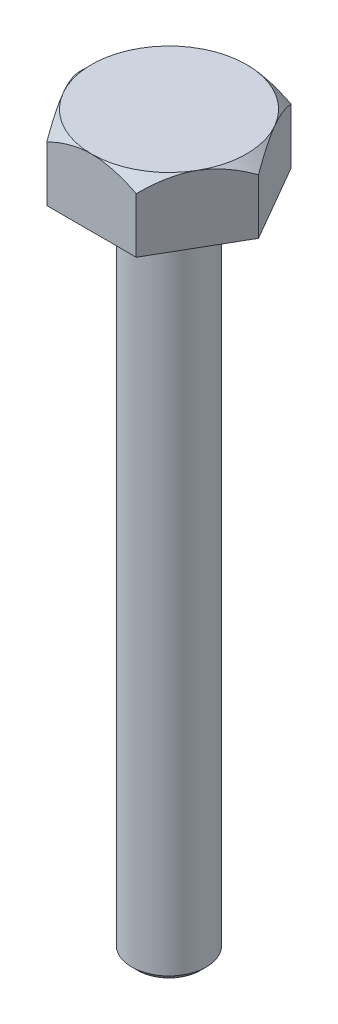
SolidWorks part; units mm, degrees
material "Plain Carbon Steel"
ref_plane "Front Plane" through (0, 0, 0) normal (0, 0, 1) x (1, 0, 0)
ref_plane "Top Plane" through (0, 0, 0) normal (0, 1, 0) x (1, 0, 0)
ref_plane "Right Plane" through (0, 0, 0) normal (1, 0, 0) x (0, 0, -1)
sketch "Hex Head Profile 104AF" plane through (0, 0, 0) normal (0, 1, 0) x (1, 0, 0)
  line L1 (30.0222, -52) -> (60.0444, 0)
  line L2 (60.0444, 0) -> (30.0222, 52)
  line L3 (30.0222, 52) -> (-30.0222, 52)
  line L4 (-30.0222, 52) -> (-60.0444, 0)
  line L5 (-60.0444, 0) -> (-30.0222, -52)
  line L6 (-30.0222, -52) -> (30.0222, -52)
  circle A0 centre (0, 0) radius 52 construction
  dimension "D1" = 104
extrude "Hex Head" add sketch "Hex Head Profile 104AF" along normal blind 45
sketch "Head Chamfer Profile" plane through (0, 45, 0) normal (0, 1, 0) x (1, 0, 0)
  line L0 (-30.0222, -52) -> (30.0222, -52) construction
  circle A0 centre (0, 0) radius 52
extrude "Head Top Chamfer 45deg" cut sketch "Head Chamfer Profile" against normal blind 45 draft 45 flip side to cut
sketch "Shank Profile Ø50" plane through (0, 0, 0) normal (0, -1, 0) x (1, 0, 0)
  circle A0 centre (0, 0) radius 25
  dimension "D1" = 50
extrude "Shank Ø50x445" add sketch "Shank Profile Ø50" along normal blind 445
chamfer "Shank End Chamfer 4x45deg" distance 4 angle 45 1 edges at (0, -445, -25)
